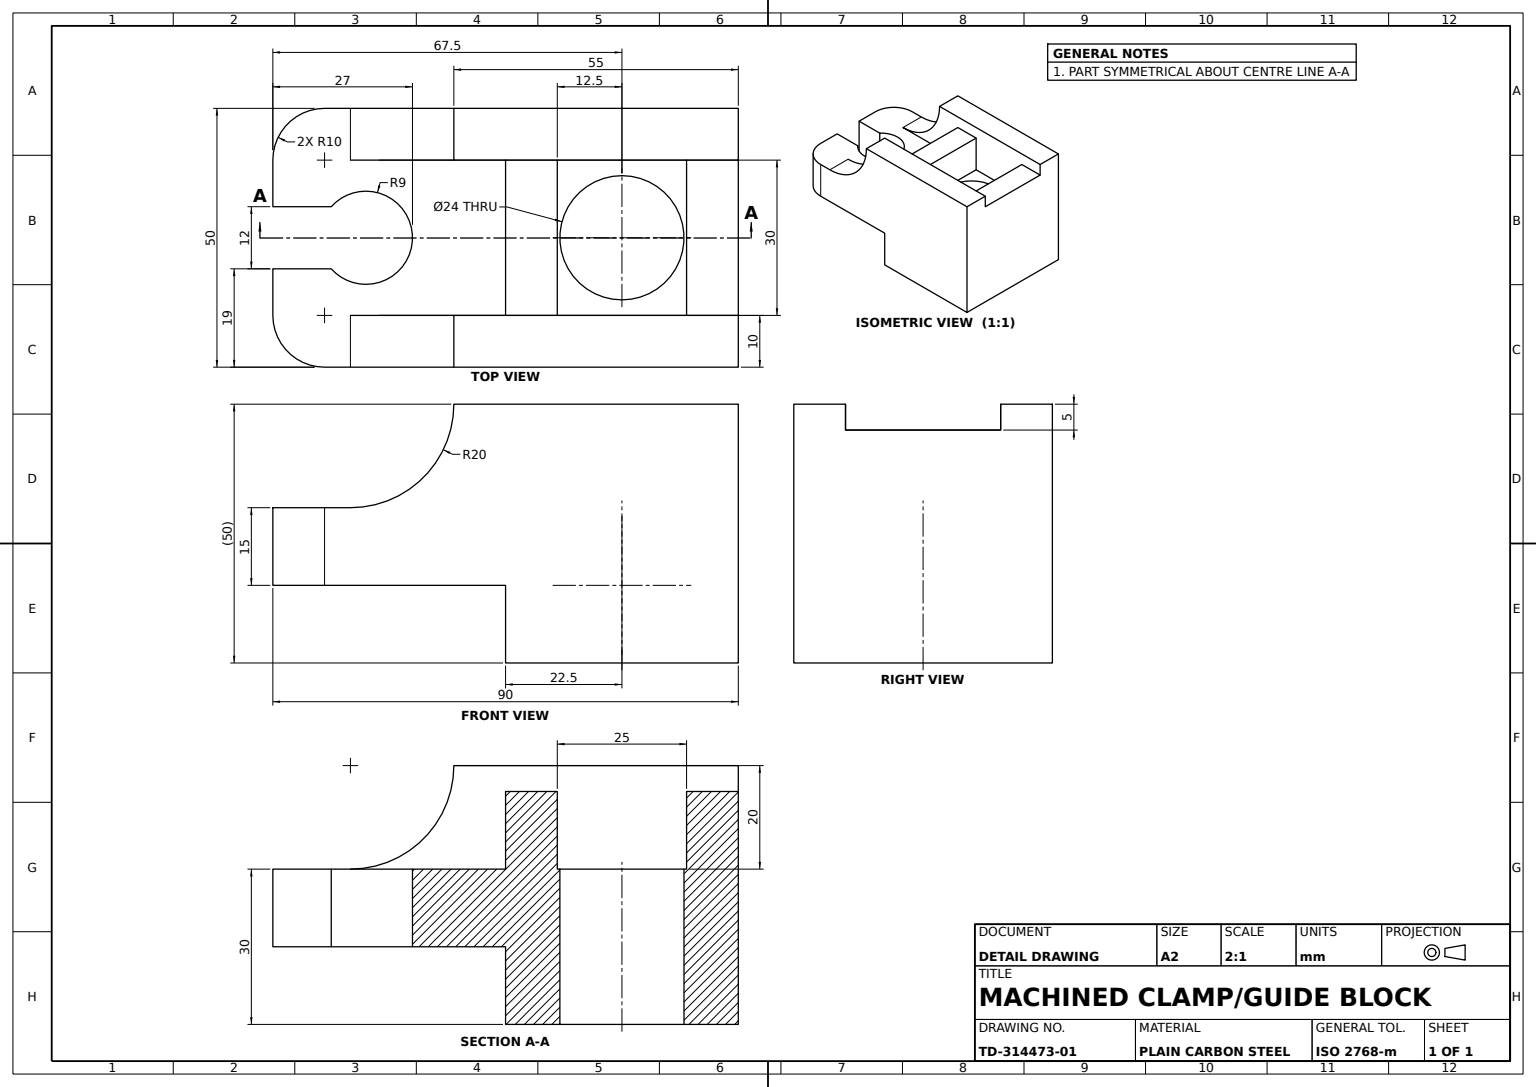
SolidWorks part; units mm, degrees
material "Plain Carbon Steel"
ref_plane "Front Plane" through (0, 0, 0) normal (0, 0, 1) x (1, 0, 0)
ref_plane "Top Plane" through (0, 0, 0) normal (0, 1, 0) x (1, 0, 0)
ref_plane "Right Plane" through (0, 0, 0) normal (1, 0, 0) x (0, 0, -1)
sketch "Base Plate Sketch" plane through (0, 0, 0) normal (0, 0, 1) x (1, 0, 0)
  line L0 (0, 0) -> (90, 0)
  line L1 (90, 0) -> (90, 15)
  line L2 (90, 15) -> (0, 15)
  line L3 (0, 15) -> (0, 0)
  dimension "D2" = 15
  dimension "D1" = 90
extrude "Base Plate" add sketch "Base Plate Sketch" against normal blind 50
sketch "Side Wall Sketch" plane through (0, 0, 0) normal (0, 0, 1) x (1, 0, 0)
  line L0 (90, 0) -> (90, -15)
  line L1 (90, -15) -> (45, -15)
  line L2 (45, -15) -> (45, 0)
  line L4 (45, 0) -> (90, 0)
  dimension "D1" = 15
  dimension "D2" = 45
  dimension "D3" = 90
extrude "Side Wall" add sketch "Side Wall Sketch" against normal blind 50
sketch "Raised Block Sketch" plane through (0, 0, 0) normal (0, 0, 1) x (1, 0, 0)
  line L0 (90, 15) -> (90, 35)
  line L1 (90, 35) -> (35, 35)
  line L2 (35, 35) -> (35, 15)
  line L3 (90, 15) -> (0, 15) construction
  line L4 (35, 15) -> (90, 15)
  dimension "D1" = 20
  dimension "D2" = 55
extrude "Raised Block" add sketch "Raised Block Sketch" against normal blind 50
sketch "Step Notch Sketch" plane through (0, 15, 0) normal (0, 1, 0) x (1, 0, 0)
  line L0 (0, 50) -> (10, 50)
  line L1 (35, 50) -> (0, 50) construction
  line L2 (10, 50) -> (10, 40)
  line L3 (0, 0) -> (10, 0)
  line L4 (35, 0) -> (0, 0) construction
  line L5 (10, 0) -> (10, 10)
  line L6 (0, 50) -> (0, 40)
  line L7 (0, 0) -> (0, 10)
  arc A0 (10, 50) -> (0, 40) centre (10, 40) ccw
  arc A1 (0, 10) -> (10, 0) centre (10, 10) ccw
  line M5 (35, 50) -> (0, 50)
  line M6 (0, 50) -> (0, 0)
  line M7 (0, 0) -> (35, 0)
  dimension "D3" = 10
  dimension "D6" = 10
  dimension "D1" = 10
  dimension "D2" = 10
  dimension "D4" = 10
  dimension "D5" = 10
  dimension "D7" = 10
  dimension "D8" = 10
extrude "Step Notch Cut" cut sketch "Step Notch Sketch" against normal blind 50 contours A0 M5 M6 | A1 M6 M7
sketch "First Rounded Lug Sketch" plane through (0, 0, 0) normal (0, 0, 1) x (1, 0, 0)
  line L0 (35, 15) -> (10, 15) construction
  line L1 (35, 35) -> (35, 15)
  line L2 (35, 15) -> (15, 15)
  arc A0 (15, 15) -> (35, 35) centre (15, 35) ccw
  dimension "D1" = 20
extrude "First Rounded Lug" add sketch "First Rounded Lug Sketch" against normal blind 10
sketch "Second Rounded Lug Sketch" plane through (0, 0, -50) normal (0, 0, -1) x (-1, 0, 0)
  line L0 (-35, 35) -> (-35, 15)
  line L1 (-35, 15) -> (-15, 15)
  arc A0 (-35, 35) -> (-15, 15) centre (-15, 35) ccw
  dimension "D1" = 20
extrude "Second Rounded Lug" add sketch "Second Rounded Lug Sketch" against normal blind 10
sketch "Slot Sketch" plane through (0, 15, 0) normal (0, 1, 0) x (1, 0, 0)
  line L0 (35, 40) -> (35, 10) construction
  line L1 (0, 40) -> (0, 10) construction
  line L2 (0, 25) -> (0, 31)
  line L3 (0, 31) -> (11.2918, 31)
  line L5 (11.2918, 19) -> (0, 19)
  line L6 (0, 19) -> (0, 25)
  arc A0 (11.2918, 19) -> (11.2918, 31) centre (18, 25) ccw
  dimension "D2" = 18
  dimension "D1" = 18
  dimension "D3" = 6
  dimension "D4" = 17
  dimension "D5" = 12
extrude "Slot Cut" cut sketch "Slot Sketch" against normal blind 15
sketch "Channel Sketch" plane through (35, 0, 0) normal (-1, 0, 0) x (0, 0, 1)
  line L0 (-40, 35) -> (-10, 35)
  line L1 (-10, 35) -> (-10, 15)
  line L2 (-10, 15) -> (-40, 15)
  line L3 (-40, 15) -> (-40, 35)
extrude "Channel Cut" cut sketch "Channel Sketch" against normal blind 60
sketch "Rail Boss Sketch" plane through (90, 0, 0) normal (1, 0, 0) x (0, 0, -1)
  line L0 (10, 35) -> (40, 35)
  line L1 (40, 35) -> (40, 15)
  line L2 (40, 15) -> (10, 15)
  line L3 (10, 15) -> (10, 35)
extrude "Rail Boss" add sketch "Rail Boss Sketch" against normal blind 10
sketch "Curved Recess Sketch" plane through (0, 35, 0) normal (0, 1, 0) x (1, 0, 0)
  line L0 (80, 40) -> (90, 40)
  line L1 (90, 50) -> (90, 0) construction
  line L2 (90, 40) -> (90, 10)
  line L3 (90, 10) -> (80, 10)
  line L4 (80, 10) -> (80, 40)
  dimension "D1" = 30
  dimension "D2" = 90
extrude "Curved Recess Cut" cut sketch "Curved Recess Sketch" against normal blind 5
sketch "Bridge Block Sketch" plane through (0, 35, 0) normal (0, 1, 0) x (1, 0, 0)
  line L1 (90, 40) -> (35, 40) construction
  line L2 (55, 40) -> (55, 10)
  line L4 (55, 10) -> (45, 10)
  line L5 (15, 10) -> (80, 10) construction
  line L6 (45, 10) -> (45, 40)
  line L7 (45, 40) -> (55, 40)
  dimension "D1" = 10
  dimension "D2" = 30
  dimension "D3" = 10
  dimension "D4" = 30
  dimension "D5" = 30
  dimension "D6" = 55
extrude "Bridge Block" add sketch "Bridge Block Sketch" against normal blind 20
sketch "Bridge Relief Sketch" plane through (0, 35, 0) normal (0, 1, 0) x (1, 0, 0)
  line L0 (45, 40) -> (55, 40)
  line L1 (55, 40) -> (55, 10)
  line L2 (55, 10) -> (45, 10)
  line L3 (45, 10) -> (45, 40)
extrude "Bridge Relief Cut" cut sketch "Bridge Relief Sketch" against normal blind 5
sketch "Bore Ø24 Sketch" plane through (0, 15, 0) normal (0, 1, 0) x (1, 0, 0)
  line L0 (80, 40) -> (80, 10) construction
  line L1 (90, 10) -> (35, 10) construction
  circle A0 centre (67.5, 25) radius 12
  dimension "D1" = 24
  dimension "D2" = 12.5
  dimension "D3" = 15
extrude "Bore Ø24" cut sketch "Bore Ø24 Sketch" against normal blind 70
